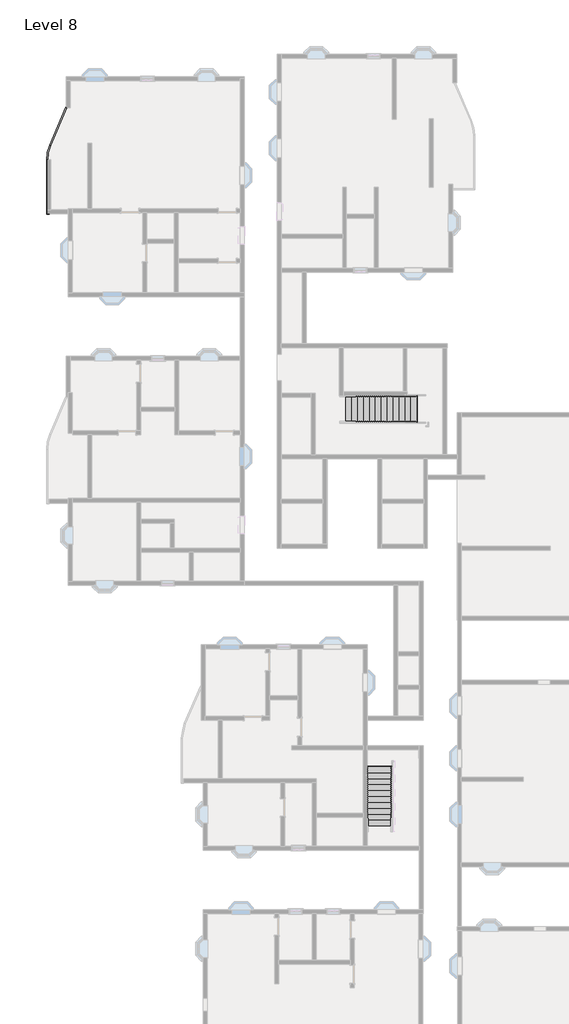
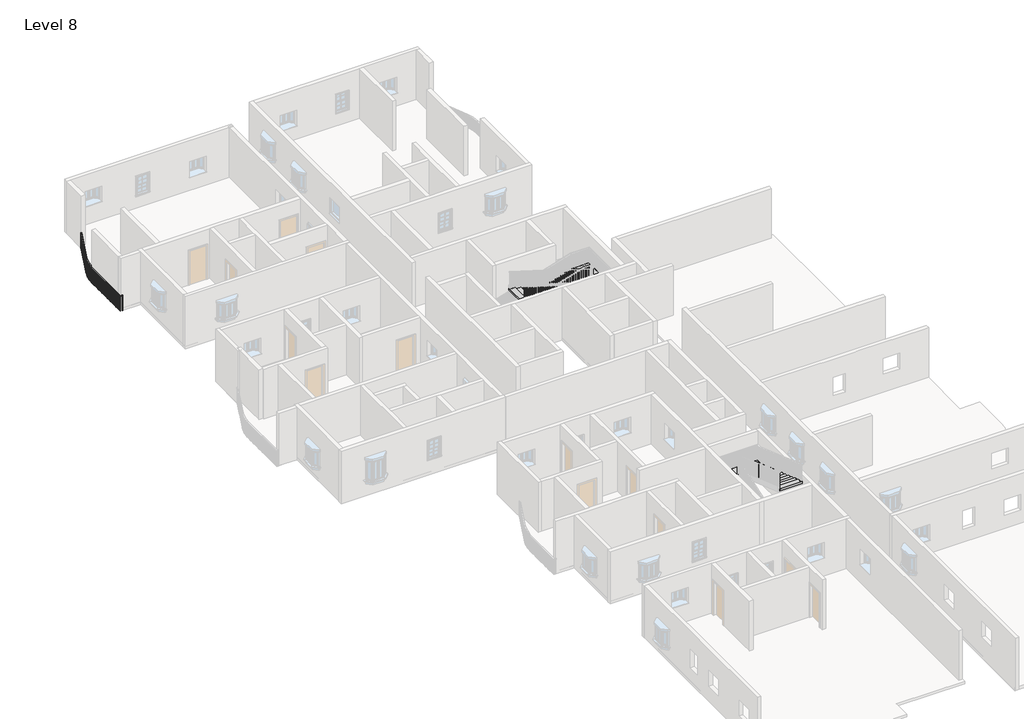
# One storey, part 12 of 14: 2 stair flights, 1 railing.
"""IFC4 building model written with IfcOpenShell, lengths in millimetres."""

from ifc_helpers import new_model, si_unit, frame, origin, place, context, project, spatial, polyline, circle_curve, outline, extrude, transform, mapped, element, save
from ifc_brep_helpers import plane_surface, cylinder_surface, revolved_surface, advanced_brep
from components import stair_flight_f068cff5, stair_flight_f74c360e

model = new_model("IFC4")

# Units and contexts
model_context = context("Model", 3, world=origin())
ifc_project = project(units=[si_unit("LENGTHUNIT", "METRE", prefix="MILLI")], contexts=[model_context])

# Site, building, storey
site = spatial("IfcSite", under=ifc_project)
building = spatial("IfcBuilding", under=site)
storey = spatial("IfcBuildingStorey", under=building, Name="Level 8", Elevation=21336.0)

# Railing
placement = place(None, origin())
element("IfcRailing", 1, ObjectType="Handrail - Rectangular", at=placement, inside=storey, context=model_context, shape_type="SolidModel", body=[
    advanced_brep(
    [(-19327.739878, 27355.8257339, 22250.4), (-19327.739878, 27355.8257339, 22199.6), (-19374.4383922, 27375.822953, 22199.6), (-19374.4383922, 27375.822953, 22250.4), (-20162.483418, 25406.4905323, 22250.4), (-20162.483418, 25406.4905323, 22199.6), (-20209.1819322, 25426.4877514, 22199.6), (-20209.1819322, 25426.4877514, 22250.4), (-20316.2891351, 24656.5948172, 22199.6), (-20316.2891351, 24656.5948172, 22250.4), (-20367.0891351, 24656.5948172, 22199.6), (-20367.0891351, 24656.5948172, 22250.4), (-20316.2891351, 21915.0583494, 22250.4), (-20316.2891351, 21915.0583494, 22199.6), (-20367.0891351, 21864.2583494, 22199.6), (-20367.0891351, 21864.2583494, 22250.4), (-20240.0891351, 21915.0583494, 22250.4), (-20240.0891351, 21864.2583494, 22250.4), (-20240.0891351, 21864.2583494, 22199.6), (-20240.0891351, 21915.0583494, 22199.6)],
    [
        (0, 1),
        (1, 2),
        (2, 3),
        (3, 0),
        (0, 4),
        (4, 5),
        (5, 1),
        (5, 6),
        (6, 2),
        (6, 7),
        (7, 3),
        (7, 4),
        (8, 5, circle_curve(frame((-18411.2891351, 24656.5948172, 22199.6), z_axis=(0.0, 0.0, -1.0), x_axis=(-0.9192620907623792, 0.3936460446736121, 0.0)), 1905.0)),
        (4, 9, circle_curve(frame((-18411.2891351, 24656.5948172, 22250.4), z_axis=(0.0, 0.0, 1.0), x_axis=(-0.9192620907623792, 0.3936460446736121, 0.0)), 1905.0)),
        (9, 8),
        (10, 6, circle_curve(frame((-18411.2891351, 24656.5948172, 22199.6), z_axis=(0.0, 0.0, -1.0), x_axis=(-0.9192620907623792, 0.3936460446736121, 0.0)), 1955.8)),
        (8, 10),
        (11, 7, circle_curve(frame((-18411.2891351, 24656.5948172, 22250.4), z_axis=(0.0, 0.0, -1.0), x_axis=(-0.9192620907623792, 0.3936460446736121, 0.0)), 1955.8)),
        (10, 11),
        (11, 9),
        (9, 12),
        (12, 13),
        (13, 8),
        (13, 14),
        (14, 10),
        (14, 15),
        (15, 11),
        (15, 12),
        (16, 17),
        (17, 18),
        (18, 19),
        (19, 16),
        (12, 16),
        (19, 13),
        (18, 14),
        (17, 15),
    ],
    [
        plane_surface(frame((-19351.0891351, 27365.8243434, 22250.4), z_axis=(0.3936460446736102, 0.91926209076238, 0.0), x_axis=(0.91926209076238, -0.3936460446736102, 0.0))),
        plane_surface(frame((-19327.739878, 27355.8257339, 22250.4), z_axis=(0.91926209076238, -0.3936460446736102, 0.0), x_axis=(-0.3936460446736102, -0.91926209076238, 0.0))),
        plane_surface(frame((-19327.739878, 27355.8257339, 22199.6), z_axis=(0.0, 0.0, -1.0), x_axis=(-0.3936460446736102, -0.91926209076238, 0.0))),
        plane_surface(frame((-19374.4383922, 27375.822953, 22199.6), z_axis=(-0.91926209076238, 0.3936460446736102, 0.0), x_axis=(-0.3936460446736102, -0.91926209076238, 0.0))),
        plane_surface(frame((-19374.4383922, 27375.822953, 22250.4), z_axis=(0.0, 0.0, 1.0), x_axis=(-0.3936460446736102, -0.91926209076238, 0.0))),
        revolved_surface(polyline([(-20162.48341800233, 25406.49053230323, 22250.4), (-20162.48341800233, 25406.49053230323, 22199.6)]), (-18411.2891351, 24656.5948172, 22250.4), (0.0, 0.0, 1.0)),
        plane_surface(frame((-18411.2891351, 24656.5948172, 22199.6), z_axis=(0.0, 0.0, -1.0), x_axis=(-0.9192620907623792, 0.3936460446736121, 0.0))),
        cylinder_surface(frame((-18411.2891351, 24656.5948172, 22250.4), z_axis=(0.0, 0.0, 1.0), x_axis=(-0.9192620907623792, 0.3936460446736121, 0.0)), 1955.8),
        plane_surface(frame((-18411.2891351, 24656.5948172, 22250.4), z_axis=(0.0, 0.0, 1.0), x_axis=(-0.9192620907623792, 0.3936460446736121, 0.0))),
        plane_surface(frame((-20316.2891351, 24656.5948172, 22250.4), z_axis=(1.0, 0.0, 0.0), x_axis=(0.0, -1.0, 0.0))),
        plane_surface(frame((-20316.2891351, 24656.5948172, 22199.6), z_axis=(0.0, 0.0, -1.0), x_axis=(0.0, -1.0, 0.0))),
        plane_surface(frame((-20367.0891351, 24656.5948172, 22199.6), z_axis=(-1.0, 0.0, 0.0), x_axis=(0.0, -1.0, 0.0))),
        plane_surface(frame((-20367.0891351, 24656.5948172, 22250.4), z_axis=(0.0, 0.0, 1.0), x_axis=(0.0, -1.0, 0.0))),
        plane_surface(frame((-20240.0891351, 21889.6583494, 22250.4), z_axis=(1.0, 0.0, 0.0), x_axis=(0.0, 1.0, 0.0))),
        plane_surface(frame((-20316.2891351, 21915.0583494, 22250.4), z_axis=(0.0, 1.0, 0.0), x_axis=(1.0, 0.0, 0.0))),
        plane_surface(frame((-20316.2891351, 21915.0583494, 22199.6), z_axis=(0.0, 0.0, -1.0), x_axis=(1.0, 0.0, 0.0))),
        plane_surface(frame((-20367.0891351, 21864.2583494, 22199.6), z_axis=(0.0, -1.0, 0.0), x_axis=(1.0, 0.0, 0.0))),
        plane_surface(frame((-20367.0891351, 21864.2583494, 22250.4), z_axis=(0.0, 0.0, 1.0), x_axis=(1.0, 0.0, 0.0))),
    ],
    [
        (0, [[1, 2, 3, 4]]),
        (1, [[-1, 5, 6, 7]]),
        (2, [[-2, -7, 8, 9]]),
        (3, [[-3, -9, 10, 11]]),
        (4, [[-4, -11, 12, -5]]),
        (5, [[13, -6, 14, 15]]),
        (6, [[16, -8, -13, 17]]),
        (7, [[18, -10, -16, 19]]),
        (8, [[-14, -12, -18, 20]]),
        (9, [[-15, 21, 22, 23]]),
        (10, [[-17, -23, 24, 25]]),
        (11, [[-19, -25, 26, 27]]),
        (12, [[-20, -27, 28, -21]]),
        (13, [[29, 30, 31, 32]]),
        (14, [[-22, 33, -32, 34]]),
        (15, [[-24, -34, -31, 35]]),
        (16, [[-26, -35, -30, 36]]),
        (17, [[-28, -36, -29, -33]]),
    ],
),
    extrude(outline(polyline([(-20351.2141351, 21922.9198172), (-20332.1641351, 21922.9198172), (-20332.1641351, 21903.8698172), (-20351.2141351, 21903.8698172), (-20351.2141351, 21922.9198172)])), frame((0.0, 0.0, 21336.0), z_axis=(0.0, 0.0, 1.0), x_axis=(1.0, 0.0, 0.0)), (0.0, 0.0, 1.0), 863.6),
    extrude(outline(polyline([(-20351.2141351, 22024.5198172), (-20332.1641351, 22024.5198172), (-20332.1641351, 22005.4698172), (-20351.2141351, 22005.4698172), (-20351.2141351, 22024.5198172)])), frame((0.0, 0.0, 21336.0), z_axis=(0.0, 0.0, 1.0), x_axis=(1.0, 0.0, 0.0)), (0.0, 0.0, 1.0), 863.6),
    extrude(outline(polyline([(-20351.2141351, 22126.1198172), (-20332.1641351, 22126.1198172), (-20332.1641351, 22107.0698172), (-20351.2141351, 22107.0698172), (-20351.2141351, 22126.1198172)])), frame((0.0, 0.0, 21336.0), z_axis=(0.0, 0.0, 1.0), x_axis=(1.0, 0.0, 0.0)), (0.0, 0.0, 1.0), 863.6),
    extrude(outline(polyline([(-20351.2141351, 22227.7198172), (-20332.1641351, 22227.7198172), (-20332.1641351, 22208.6698172), (-20351.2141351, 22208.6698172), (-20351.2141351, 22227.7198172)])), frame((0.0, 0.0, 21336.0), z_axis=(0.0, 0.0, 1.0), x_axis=(1.0, 0.0, 0.0)), (0.0, 0.0, 1.0), 863.6),
    extrude(outline(polyline([(-20351.2141351, 22329.3198172), (-20332.1641351, 22329.3198172), (-20332.1641351, 22310.2698172), (-20351.2141351, 22310.2698172), (-20351.2141351, 22329.3198172)])), frame((0.0, 0.0, 21336.0), z_axis=(0.0, 0.0, 1.0), x_axis=(1.0, 0.0, 0.0)), (0.0, 0.0, 1.0), 863.6),
    extrude(outline(polyline([(-20351.2141351, 22430.9198172), (-20332.1641351, 22430.9198172), (-20332.1641351, 22411.8698172), (-20351.2141351, 22411.8698172), (-20351.2141351, 22430.9198172)])), frame((0.0, 0.0, 21336.0), z_axis=(0.0, 0.0, 1.0), x_axis=(1.0, 0.0, 0.0)), (0.0, 0.0, 1.0), 863.6),
    extrude(outline(polyline([(-20351.2141351, 22532.5198172), (-20332.1641351, 22532.5198172), (-20332.1641351, 22513.4698172), (-20351.2141351, 22513.4698172), (-20351.2141351, 22532.5198172)])), frame((0.0, 0.0, 21336.0), z_axis=(0.0, 0.0, 1.0), x_axis=(1.0, 0.0, 0.0)), (0.0, 0.0, 1.0), 863.6),
    extrude(outline(polyline([(-20351.2141351, 22634.1198172), (-20332.1641351, 22634.1198172), (-20332.1641351, 22615.0698172), (-20351.2141351, 22615.0698172), (-20351.2141351, 22634.1198172)])), frame((0.0, 0.0, 21336.0), z_axis=(0.0, 0.0, 1.0), x_axis=(1.0, 0.0, 0.0)), (0.0, 0.0, 1.0), 863.6),
    extrude(outline(polyline([(-20351.2141351, 22735.7198172), (-20332.1641351, 22735.7198172), (-20332.1641351, 22716.6698172), (-20351.2141351, 22716.6698172), (-20351.2141351, 22735.7198172)])), frame((0.0, 0.0, 21336.0), z_axis=(0.0, 0.0, 1.0), x_axis=(1.0, 0.0, 0.0)), (0.0, 0.0, 1.0), 863.6),
    extrude(outline(polyline([(-20351.2141351, 22837.3198172), (-20332.1641351, 22837.3198172), (-20332.1641351, 22818.2698172), (-20351.2141351, 22818.2698172), (-20351.2141351, 22837.3198172)])), frame((0.0, 0.0, 21336.0), z_axis=(0.0, 0.0, 1.0), x_axis=(1.0, 0.0, 0.0)), (0.0, 0.0, 1.0), 863.6),
    extrude(outline(polyline([(-20351.2141351, 22938.9198172), (-20332.1641351, 22938.9198172), (-20332.1641351, 22919.8698172), (-20351.2141351, 22919.8698172), (-20351.2141351, 22938.9198172)])), frame((0.0, 0.0, 21336.0), z_axis=(0.0, 0.0, 1.0), x_axis=(1.0, 0.0, 0.0)), (0.0, 0.0, 1.0), 863.6),
    extrude(outline(polyline([(-20351.2141351, 23040.5198172), (-20332.1641351, 23040.5198172), (-20332.1641351, 23021.4698172), (-20351.2141351, 23021.4698172), (-20351.2141351, 23040.5198172)])), frame((0.0, 0.0, 21336.0), z_axis=(0.0, 0.0, 1.0), x_axis=(1.0, 0.0, 0.0)), (0.0, 0.0, 1.0), 863.6),
    extrude(outline(polyline([(-20351.2141351, 23142.1198172), (-20332.1641351, 23142.1198172), (-20332.1641351, 23123.0698172), (-20351.2141351, 23123.0698172), (-20351.2141351, 23142.1198172)])), frame((0.0, 0.0, 21336.0), z_axis=(0.0, 0.0, 1.0), x_axis=(1.0, 0.0, 0.0)), (0.0, 0.0, 1.0), 863.6),
    extrude(outline(polyline([(-20351.2141351, 23243.7198172), (-20332.1641351, 23243.7198172), (-20332.1641351, 23224.6698172), (-20351.2141351, 23224.6698172), (-20351.2141351, 23243.7198172)])), frame((0.0, 0.0, 21336.0), z_axis=(0.0, 0.0, 1.0), x_axis=(1.0, 0.0, 0.0)), (0.0, 0.0, 1.0), 863.6),
    extrude(outline(polyline([(-20351.2141351, 23345.3198172), (-20332.1641351, 23345.3198172), (-20332.1641351, 23326.2698172), (-20351.2141351, 23326.2698172), (-20351.2141351, 23345.3198172)])), frame((0.0, 0.0, 21336.0), z_axis=(0.0, 0.0, 1.0), x_axis=(1.0, 0.0, 0.0)), (0.0, 0.0, 1.0), 863.6),
    extrude(outline(polyline([(-20351.2141351, 23446.9198172), (-20332.1641351, 23446.9198172), (-20332.1641351, 23427.8698172), (-20351.2141351, 23427.8698172), (-20351.2141351, 23446.9198172)])), frame((0.0, 0.0, 21336.0), z_axis=(0.0, 0.0, 1.0), x_axis=(1.0, 0.0, 0.0)), (0.0, 0.0, 1.0), 863.6),
    extrude(outline(polyline([(-20351.2141351, 23548.5198172), (-20332.1641351, 23548.5198172), (-20332.1641351, 23529.4698172), (-20351.2141351, 23529.4698172), (-20351.2141351, 23548.5198172)])), frame((0.0, 0.0, 21336.0), z_axis=(0.0, 0.0, 1.0), x_axis=(1.0, 0.0, 0.0)), (0.0, 0.0, 1.0), 863.6),
    extrude(outline(polyline([(-20351.2141351, 23650.1198172), (-20332.1641351, 23650.1198172), (-20332.1641351, 23631.0698172), (-20351.2141351, 23631.0698172), (-20351.2141351, 23650.1198172)])), frame((0.0, 0.0, 21336.0), z_axis=(0.0, 0.0, 1.0), x_axis=(1.0, 0.0, 0.0)), (0.0, 0.0, 1.0), 863.6),
    extrude(outline(polyline([(-20351.2141351, 23751.7198172), (-20332.1641351, 23751.7198172), (-20332.1641351, 23732.6698172), (-20351.2141351, 23732.6698172), (-20351.2141351, 23751.7198172)])), frame((0.0, 0.0, 21336.0), z_axis=(0.0, 0.0, 1.0), x_axis=(1.0, 0.0, 0.0)), (0.0, 0.0, 1.0), 863.6),
    extrude(outline(polyline([(-20351.2141351, 23853.3198172), (-20332.1641351, 23853.3198172), (-20332.1641351, 23834.2698172), (-20351.2141351, 23834.2698172), (-20351.2141351, 23853.3198172)])), frame((0.0, 0.0, 21336.0), z_axis=(0.0, 0.0, 1.0), x_axis=(1.0, 0.0, 0.0)), (0.0, 0.0, 1.0), 863.6),
    extrude(outline(polyline([(-20351.2141351, 23954.9198172), (-20332.1641351, 23954.9198172), (-20332.1641351, 23935.8698172), (-20351.2141351, 23935.8698172), (-20351.2141351, 23954.9198172)])), frame((0.0, 0.0, 21336.0), z_axis=(0.0, 0.0, 1.0), x_axis=(1.0, 0.0, 0.0)), (0.0, 0.0, 1.0), 863.6),
    extrude(outline(polyline([(-20351.2141351, 24056.5198172), (-20332.1641351, 24056.5198172), (-20332.1641351, 24037.4698172), (-20351.2141351, 24037.4698172), (-20351.2141351, 24056.5198172)])), frame((0.0, 0.0, 21336.0), z_axis=(0.0, 0.0, 1.0), x_axis=(1.0, 0.0, 0.0)), (0.0, 0.0, 1.0), 863.6),
    extrude(outline(polyline([(-20351.2141351, 24158.1198172), (-20332.1641351, 24158.1198172), (-20332.1641351, 24139.0698172), (-20351.2141351, 24139.0698172), (-20351.2141351, 24158.1198172)])), frame((0.0, 0.0, 21336.0), z_axis=(0.0, 0.0, 1.0), x_axis=(1.0, 0.0, 0.0)), (0.0, 0.0, 1.0), 863.6),
    extrude(outline(polyline([(-20351.2141351, 24259.7198172), (-20332.1641351, 24259.7198172), (-20332.1641351, 24240.6698172), (-20351.2141351, 24240.6698172), (-20351.2141351, 24259.7198172)])), frame((0.0, 0.0, 21336.0), z_axis=(0.0, 0.0, 1.0), x_axis=(1.0, 0.0, 0.0)), (0.0, 0.0, 1.0), 863.6),
    extrude(outline(polyline([(-20351.2141351, 24361.3198172), (-20332.1641351, 24361.3198172), (-20332.1641351, 24342.2698172), (-20351.2141351, 24342.2698172), (-20351.2141351, 24361.3198172)])), frame((0.0, 0.0, 21336.0), z_axis=(0.0, 0.0, 1.0), x_axis=(1.0, 0.0, 0.0)), (0.0, 0.0, 1.0), 863.6),
    extrude(outline(polyline([(-20351.2141351, 24462.9198172), (-20332.1641351, 24462.9198172), (-20332.1641351, 24443.8698172), (-20351.2141351, 24443.8698172), (-20351.2141351, 24462.9198172)])), frame((0.0, 0.0, 21336.0), z_axis=(0.0, 0.0, 1.0), x_axis=(1.0, 0.0, 0.0)), (0.0, 0.0, 1.0), 863.6),
    extrude(outline(polyline([(-20351.2141351, 24564.5198172), (-20332.1641351, 24564.5198172), (-20332.1641351, 24545.4698172), (-20351.2141351, 24545.4698172), (-20351.2141351, 24564.5198172)])), frame((0.0, 0.0, 21336.0), z_axis=(0.0, 0.0, 1.0), x_axis=(1.0, 0.0, 0.0)), (0.0, 0.0, 1.0), 863.6),
    extrude(outline(polyline([(-20349.6005818, 24736.2720848), (-20330.5630441, 24735.5831307), (-20331.2519982, 24716.545593), (-20350.289536, 24717.2345471), (-20349.6005818, 24736.2720848)])), frame((0.0, 0.0, 21336.0), z_axis=(0.0, 0.0, 1.0), x_axis=(1.0, 0.0, 0.0)), (0.0, 0.0, 1.0), 863.6),
    extrude(outline(polyline([(-20342.724955, 24838.1310534), (-20323.750023, 24836.4415402), (-20325.4395363, 24817.4666081), (-20344.4144683, 24819.1561214), (-20342.724955, 24838.1310534)])), frame((0.0, 0.0, 21336.0), z_axis=(0.0, 0.0, 1.0), x_axis=(1.0, 0.0, 0.0)), (0.0, 0.0, 1.0), 863.6),
    extrude(outline(polyline([(-20330.5003254, 24939.4872677), (-20311.6405491, 24936.8018743), (-20314.3259425, 24917.942098), (-20333.1857188, 24920.6274914), (-20330.5003254, 24939.4872677)])), frame((0.0, 0.0, 21336.0), z_axis=(0.0, 0.0, 1.0), x_axis=(1.0, 0.0, 0.0)), (0.0, 0.0, 1.0), 863.6),
    extrude(outline(polyline([(-20312.9605484, 25040.0600272), (-20294.2681589, 25036.3861907), (-20297.9419954, 25017.6938012), (-20316.6343849, 25021.3676377), (-20312.9605484, 25040.0600272)])), frame((0.0, 0.0, 21336.0), z_axis=(0.0, 0.0, 1.0), x_axis=(1.0, 0.0, 0.0)), (0.0, 0.0, 1.0), 863.6),
    extrude(outline(polyline([(-20290.1541995, 25139.5708014), (-20271.6809643, 25134.9186963), (-20276.3330693, 25116.4454611), (-20294.8063045, 25121.0975662), (-20290.1541995, 25139.5708014)])), frame((0.0, 0.0, 21336.0), z_axis=(0.0, 0.0, 1.0), x_axis=(1.0, 0.0, 0.0)), (0.0, 0.0, 1.0), 863.6),
    extrude(outline(polyline([(-20262.1444395, 25237.7440008), (-20243.9415192, 25232.1265109), (-20249.5590091, 25213.9235906), (-20267.7619294, 25219.5410805), (-20262.1444395, 25237.7440008)])), frame((0.0, 0.0, 21336.0), z_axis=(0.0, 0.0, 1.0), x_axis=(1.0, 0.0, 0.0)), (0.0, 0.0, 1.0), 863.6),
    extrude(outline(polyline([(-20229.0088399, 25334.3077402), (-20211.1266465, 25327.7404228), (-20217.693964, 25309.8582293), (-20235.5761574, 25316.4255468), (-20229.0088399, 25334.3077402)])), frame((0.0, 0.0, 21336.0), z_axis=(0.0, 0.0, 1.0), x_axis=(1.0, 0.0, 0.0)), (0.0, 0.0, 1.0), 863.6),
    extrude(outline(polyline([(-20155.9843907, 25510.389225), (-20138.4724479, 25502.8902678), (-20145.9714051, 25485.378325), (-20163.4833479, 25492.8772822), (-20155.9843907, 25510.389225)])), frame((0.0, 0.0, 21336.0), z_axis=(0.0, 0.0, 1.0), x_axis=(1.0, 0.0, 0.0)), (0.0, 0.0, 1.0), 863.6),
    extrude(outline(polyline([(-20115.9899526, 25603.7862534), (-20098.4780098, 25596.2872963), (-20105.9769669, 25578.7753534), (-20123.4889098, 25586.2743106), (-20115.9899526, 25603.7862534)])), frame((0.0, 0.0, 21336.0), z_axis=(0.0, 0.0, 1.0), x_axis=(1.0, 0.0, 0.0)), (0.0, 0.0, 1.0), 863.6),
    extrude(outline(polyline([(-20075.9955145, 25697.1832818), (-20058.4835716, 25689.6843247), (-20065.9825288, 25672.1723818), (-20083.4944716, 25679.671339), (-20075.9955145, 25697.1832818)])), frame((0.0, 0.0, 21336.0), z_axis=(0.0, 0.0, 1.0), x_axis=(1.0, 0.0, 0.0)), (0.0, 0.0, 1.0), 863.6),
    extrude(outline(polyline([(-20036.0010763, 25790.5803103), (-20018.4891335, 25783.0813531), (-20025.9880906, 25765.5694103), (-20043.5000335, 25773.0683674), (-20036.0010763, 25790.5803103)])), frame((0.0, 0.0, 21336.0), z_axis=(0.0, 0.0, 1.0), x_axis=(1.0, 0.0, 0.0)), (0.0, 0.0, 1.0), 863.6),
    extrude(outline(polyline([(-19996.0066382, 25883.9773387), (-19978.4946954, 25876.4783815), (-19985.9936525, 25858.9664387), (-20003.5055953, 25866.4653958), (-19996.0066382, 25883.9773387)])), frame((0.0, 0.0, 21336.0), z_axis=(0.0, 0.0, 1.0), x_axis=(1.0, 0.0, 0.0)), (0.0, 0.0, 1.0), 863.6),
    extrude(outline(polyline([(-19956.0122, 25977.3743671), (-19938.5002572, 25969.8754099), (-19945.9992144, 25952.3634671), (-19963.5111572, 25959.8624243), (-19956.0122, 25977.3743671)])), frame((0.0, 0.0, 21336.0), z_axis=(0.0, 0.0, 1.0), x_axis=(1.0, 0.0, 0.0)), (0.0, 0.0, 1.0), 863.6),
    extrude(outline(polyline([(-19916.0177619, 26070.7713955), (-19898.5058191, 26063.2724384), (-19906.0047762, 26045.7604955), (-19923.5167191, 26053.2594527), (-19916.0177619, 26070.7713955)])), frame((0.0, 0.0, 21336.0), z_axis=(0.0, 0.0, 1.0), x_axis=(1.0, 0.0, 0.0)), (0.0, 0.0, 1.0), 863.6),
    extrude(outline(polyline([(-19876.0233238, 26164.1684239), (-19858.5113809, 26156.6694668), (-19866.0103381, 26139.157524), (-19883.5222809, 26146.6564811), (-19876.0233238, 26164.1684239)])), frame((0.0, 0.0, 21336.0), z_axis=(0.0, 0.0, 1.0), x_axis=(1.0, 0.0, 0.0)), (0.0, 0.0, 1.0), 863.6),
    extrude(outline(polyline([(-19836.0288856, 26257.5654524), (-19818.5169428, 26250.0664952), (-19826.0159, 26232.5545524), (-19843.5278428, 26240.0535095), (-19836.0288856, 26257.5654524)])), frame((0.0, 0.0, 21336.0), z_axis=(0.0, 0.0, 1.0), x_axis=(1.0, 0.0, 0.0)), (0.0, 0.0, 1.0), 863.6),
    extrude(outline(polyline([(-19796.0344475, 26350.9624808), (-19778.5225047, 26343.4635236), (-19786.0214618, 26325.9515808), (-19803.5334046, 26333.450538), (-19796.0344475, 26350.9624808)])), frame((0.0, 0.0, 21336.0), z_axis=(0.0, 0.0, 1.0), x_axis=(1.0, 0.0, 0.0)), (0.0, 0.0, 1.0), 863.6),
    extrude(outline(polyline([(-19756.0400094, 26444.3595092), (-19738.5280665, 26436.860552), (-19746.0270237, 26419.3486092), (-19763.5389665, 26426.8475664), (-19756.0400094, 26444.3595092)])), frame((0.0, 0.0, 21336.0), z_axis=(0.0, 0.0, 1.0), x_axis=(1.0, 0.0, 0.0)), (0.0, 0.0, 1.0), 863.6),
    extrude(outline(polyline([(-19716.0455712, 26537.7565376), (-19698.5336284, 26530.2575805), (-19706.0325855, 26512.7456376), (-19723.5445284, 26520.2445948), (-19716.0455712, 26537.7565376)])), frame((0.0, 0.0, 21336.0), z_axis=(0.0, 0.0, 1.0), x_axis=(1.0, 0.0, 0.0)), (0.0, 0.0, 1.0), 863.6),
    extrude(outline(polyline([(-19676.0511331, 26631.153566), (-19658.5391902, 26623.6546089), (-19666.0381474, 26606.1426661), (-19683.5500902, 26613.6416232), (-19676.0511331, 26631.153566)])), frame((0.0, 0.0, 21336.0), z_axis=(0.0, 0.0, 1.0), x_axis=(1.0, 0.0, 0.0)), (0.0, 0.0, 1.0), 863.6),
    extrude(outline(polyline([(-19636.0566949, 26724.5505945), (-19618.5447521, 26717.0516373), (-19626.0437093, 26699.5396945), (-19643.5556521, 26707.0386516), (-19636.0566949, 26724.5505945)])), frame((0.0, 0.0, 21336.0), z_axis=(0.0, 0.0, 1.0), x_axis=(1.0, 0.0, 0.0)), (0.0, 0.0, 1.0), 863.6),
    extrude(outline(polyline([(-19596.0622568, 26817.9476229), (-19578.550314, 26810.4486657), (-19586.0492711, 26792.9367229), (-19603.561214, 26800.4356801), (-19596.0622568, 26817.9476229)])), frame((0.0, 0.0, 21336.0), z_axis=(0.0, 0.0, 1.0), x_axis=(1.0, 0.0, 0.0)), (0.0, 0.0, 1.0), 863.6),
    extrude(outline(polyline([(-19556.0678187, 26911.3446513), (-19538.5558758, 26903.8456942), (-19546.054833, 26886.3337513), (-19563.5667758, 26893.8327085), (-19556.0678187, 26911.3446513)])), frame((0.0, 0.0, 21336.0), z_axis=(0.0, 0.0, 1.0), x_axis=(1.0, 0.0, 0.0)), (0.0, 0.0, 1.0), 863.6),
    extrude(outline(polyline([(-19516.0733805, 27004.7416797), (-19498.5614377, 26997.2427226), (-19506.0603948, 26979.7307797), (-19523.5723377, 26987.2297369), (-19516.0733805, 27004.7416797)])), frame((0.0, 0.0, 21336.0), z_axis=(0.0, 0.0, 1.0), x_axis=(1.0, 0.0, 0.0)), (0.0, 0.0, 1.0), 863.6),
    extrude(outline(polyline([(-19476.0789424, 27098.1387082), (-19458.5669996, 27090.639751), (-19466.0659567, 27073.1278082), (-19483.5778995, 27080.6267653), (-19476.0789424, 27098.1387082)])), frame((0.0, 0.0, 21336.0), z_axis=(0.0, 0.0, 1.0), x_axis=(1.0, 0.0, 0.0)), (0.0, 0.0, 1.0), 863.6),
    extrude(outline(polyline([(-19436.0845042, 27191.5357366), (-19418.5725614, 27184.0367794), (-19426.0715186, 27166.5248366), (-19443.5834614, 27174.0237937), (-19436.0845042, 27191.5357366)])), frame((0.0, 0.0, 21336.0), z_axis=(0.0, 0.0, 1.0), x_axis=(1.0, 0.0, 0.0)), (0.0, 0.0, 1.0), 863.6),
    extrude(outline(polyline([(-19396.0900661, 27284.932765), (-19378.5781233, 27277.4338078), (-19386.0770804, 27259.921865), (-19403.5890233, 27267.4208222), (-19396.0900661, 27284.932765)])), frame((0.0, 0.0, 21336.0), z_axis=(0.0, 0.0, 1.0), x_axis=(1.0, 0.0, 0.0)), (0.0, 0.0, 1.0), 863.6),
    extrude(outline(polyline([(-20351.2141351, 21899.1833494), (-20332.1641351, 21899.1833494), (-20332.1641351, 21880.1333494), (-20351.2141351, 21880.1333494), (-20351.2141351, 21899.1833494)])), frame((0.0, 0.0, 21336.0), z_axis=(0.0, 0.0, 1.0), x_axis=(1.0, 0.0, 0.0)), (0.0, 0.0, 1.0), 863.6),
    extrude(outline(polyline([(-20351.2141351, 24666.1198172), (-20332.1641351, 24666.1198172), (-20332.1641351, 24647.0698172), (-20351.2141351, 24647.0698172), (-20351.2141351, 24666.1198172)])), frame((0.0, 0.0, 21336.0), z_axis=(0.0, 0.0, 1.0), x_axis=(1.0, 0.0, 0.0)), (0.0, 0.0, 1.0), 863.6),
    extrude(outline(polyline([(-20190.839168, 25428.9945919), (-20173.3272251, 25421.4956347), (-20180.8261823, 25403.9836919), (-20198.3381251, 25411.482649), (-20190.839168, 25428.9945919)])), frame((0.0, 0.0, 21336.0), z_axis=(0.0, 0.0, 1.0), x_axis=(1.0, 0.0, 0.0)), (0.0, 0.0, 1.0), 863.6),
    extrude(outline(polyline([(-20259.1391351, 21880.1333494), (-20259.1391351, 21899.1833494), (-20240.0891351, 21899.1833494), (-20240.0891351, 21880.1333494), (-20259.1391351, 21880.1333494)])), frame((0.0, 0.0, 21336.0), z_axis=(0.0, 0.0, 1.0), x_axis=(1.0, 0.0, 0.0)), (0.0, 0.0, 1.0), 863.6),
    extrude(outline(polyline([(-19359.8451065, 27369.573822), (-19342.3331637, 27362.0748648), (-19349.8321209, 27344.562922), (-19367.3440637, 27352.0618792), (-19359.8451065, 27369.573822)])), frame((0.0, 0.0, 21336.0), z_axis=(0.0, 0.0, 1.0), x_axis=(1.0, 0.0, 0.0)), (0.0, 0.0, 1.0), 863.6),
])

# Stair flights
stair_flight_shape = stair_flight_f068cff5(model_context)
element("IfcStairFlight", 2, ObjectType="2\" Tread 1\" Nosing 1/4\" Riser", at=placement, inside=storey, context=model_context, shape_type="MappedRepresentation", body=[
    mapped(stair_flight_shape, transform((0.0, 0.0, 0.0), x_axis=(1.0, 0.0, 0.0), y_axis=(0.0, 1.0, 0.0), z_axis=(0.0, 0.0, 1.0))),
])
stair_flight_2_shape = stair_flight_f74c360e(model_context)
element("IfcStairFlight", 3, ObjectType="2\" Tread 1\" Nosing 1/4\" Riser", at=placement, inside=storey, context=model_context, shape_type="MappedRepresentation", body=[
    mapped(stair_flight_2_shape, transform((0.0, 0.0, 0.0), x_axis=(1.0, 0.0, 0.0), y_axis=(0.0, 1.0, 0.0), z_axis=(0.0, 0.0, 1.0))),
])

save(model, "model.ifc")

# Revit data of these elements
# Type "Handrail - Rectangular"
#   Assembly Code = "C2010400"
#   built-in parameter 1008612 = 0.0416667 (stored number, unit not read)
#   built-in parameter 1008611 = 0.0416667 (stored number, unit not read)
#   built-in parameter 1008609 = 0.333333 (stored number, unit not read)
#   built-in parameter 1008604 = 0.166667 (stored number, unit not read)
#   built-in parameter 1008603 = 0.166667 (stored number, unit not read)
#   Railing Height = 3' - 0"
#   built-in parameter 1008630 = 2
#   built-in parameter 1008610 = 2
#   built-in parameter 1008618 = Baluster - Square : 3/4"
# Element 1 (IfcRailing, "Handrail - Rectangular")
#   Phase Created = New Construction
# Elements 2, 3 (IfcStairFlight, "2\" Tread 1\" Nosing 1/4\" Riser")
#   Phase Created = New Construction
